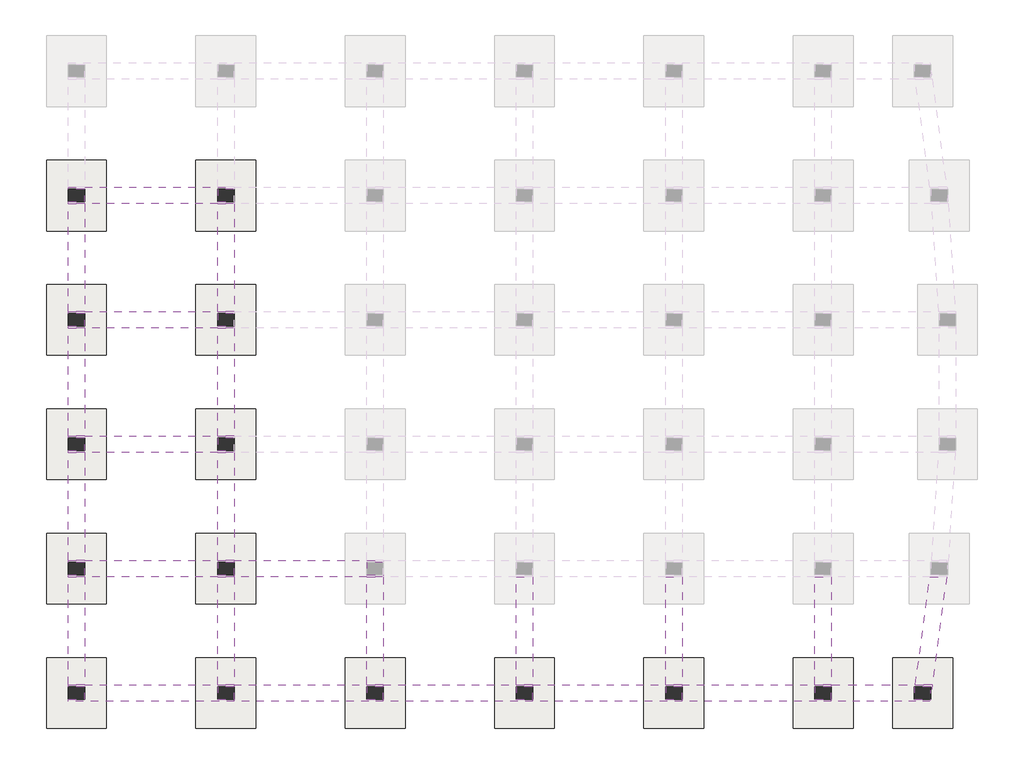
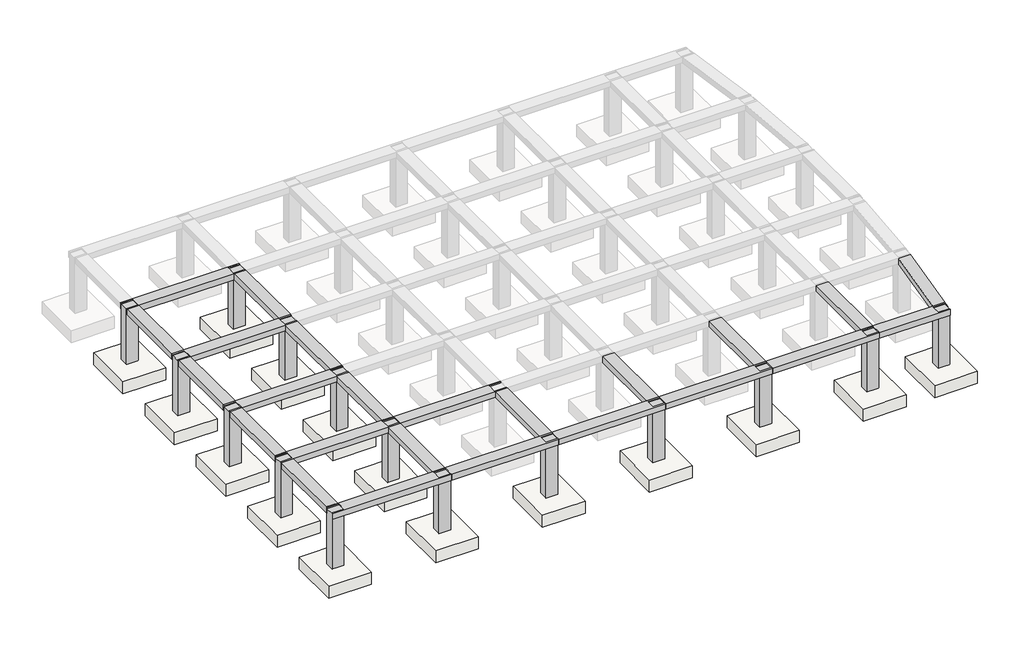
# One storey, part 1 of 3: 24 beams, 15 columns, 15 slabs.
"""IFC4 building model written with IfcOpenShell, lengths in millimetres."""

from ifc_helpers import new_model, si_unit, frame, origin, place, context, project, spatial, polyline, outline, extrude, faceted_brep, element, save

model = new_model("IFC4")

# Units and contexts
model_context = context("Model", 3, world=origin())
ifc_project = project(units=[si_unit("LENGTHUNIT", "METRE", prefix="MILLI")], contexts=[model_context])

# Site, building, storey
site = spatial("IfcSite", under=ifc_project)
building = spatial("IfcBuilding", under=site)
storey = spatial("IfcBuildingStorey", under=building, Elevation=-2999.978125)

# Beams
placement = place(None, origin())
element("IfcBeam", 1, ObjectType="Concrete-Rectangular Beam : 2' x2'", at=placement, inside=storey, context=model_context, shape_type="Brep", body=[
    faceted_brep([(-16619.274232, -2891.2168778, 48.021875), (-17228.874232, -2891.2168778, 48.021875), (-22105.674232, -2891.2168778, 48.021875), (-22715.274232, -2891.2168778, 48.021875), (-22715.274232, -2967.4168778, 48.021875), (-22105.674232, -2967.4168778, 48.021875), (-22105.674232, -3424.6168778, 48.021875), (-22715.274232, -3424.6168778, 48.021875), (-22715.274232, -3500.8168778, 48.021875), (-16619.274232, -3500.8168778, 48.021875), (-16619.274232, -3424.6168778, 48.021875), (-17228.874232, -3424.6168778, 48.021875), (-17228.874232, -2967.4168778, 48.021875), (-16619.274232, -2967.4168778, 48.021875), (-22715.274232, -3500.8168778, -256.778125), (-16619.274232, -3500.8168778, -256.778125), (-17228.874232, -3424.6168778, -256.778125), (-16619.274232, -3424.6168778, -256.778125), (-22715.274232, -3424.6168778, -256.778125), (-22105.674232, -3424.6168778, -256.778125), (-22105.674232, -2967.4168778, -256.778125), (-22715.274232, -2967.4168778, -256.778125), (-22715.274232, -2891.2168778, -256.778125), (-22105.674232, -2891.2168778, -256.778125), (-17228.874232, -2891.2168778, -256.778125), (-16619.274232, -2891.2168778, -256.778125), (-16619.274232, -2967.4168778, -256.778125), (-17228.874232, -2967.4168778, -256.778125)], [[[0, 1, 2, 3, 4, 5, 6, 7, 8, 9, 10, 11, 12, 13]], [[8, 14, 15, 9]], [[16, 17, 15, 14, 18, 19, 20, 21, 22, 23, 24, 25, 26, 27]], [[22, 3, 2, 1, 0, 25, 24, 23]], [[20, 19, 6, 5]], [[19, 18, 7, 6]], [[21, 20, 5, 4]], [[11, 10, 17, 16]], [[11, 16, 27, 12]], [[12, 27, 26, 13]], [[14, 8, 7, 18]], [[9, 15, 17, 10]], [[3, 22, 21, 4]], [[25, 0, 13, 26]]]),
])
element("IfcBeam", 2, ObjectType="Concrete-Rectangular Beam : 2' x2'", at=placement, inside=storey, context=model_context, shape_type="Brep", body=[
    faceted_brep([(-16619.274232, -2891.2168778, 48.021875), (-16619.274232, -2967.4168778, 48.021875), (-16619.274232, -3424.6168778, 48.021875), (-16619.274232, -3500.8168778, 48.021875), (-11132.874232, -3500.8168778, 48.021875), (-11132.874232, -3424.6168778, 48.021875), (-11742.474232, -3424.6168778, 48.021875), (-11742.474232, -2967.4168778, 48.021875), (-11132.874232, -2967.4168778, 48.021875), (-11132.874232, -2891.2168778, 48.021875), (-11742.474232, -2891.2168778, 48.021875), (-11132.874232, -3500.8168778, -256.778125), (-16619.274232, -3500.8168778, -256.778125), (-16619.274232, -3424.6168778, -256.778125), (-16619.274232, -2967.4168778, -256.778125), (-16619.274232, -2891.2168778, -256.778125), (-11742.474232, -2891.2168778, -256.778125), (-11132.874232, -2891.2168778, -256.778125), (-11132.874232, -2967.4168778, -256.778125), (-11742.474232, -2967.4168778, -256.778125), (-11742.474232, -3424.6168778, -256.778125), (-11132.874232, -3424.6168778, -256.778125)], [[[0, 1, 2, 3, 4, 5, 6, 7, 8, 9, 10]], [[11, 4, 3, 12]], [[12, 13, 14, 15, 16, 17, 18, 19, 20, 21, 11]], [[15, 0, 10, 9, 17, 16]], [[3, 2, 1, 0, 15, 14, 13, 12]], [[6, 5, 21, 20]], [[6, 20, 19, 7]], [[7, 19, 18, 8]], [[4, 11, 21, 5]], [[17, 9, 8, 18]]]),
])
element("IfcBeam", 3, ObjectType="Concrete-Rectangular Beam : 2' x2'", at=placement, inside=storey, context=model_context, shape_type="Brep", body=[
    faceted_brep([(-5646.474232, -2891.2168778, 48.021875), (-6256.074232, -2891.2168778, 48.021875), (-11132.874232, -2891.2168778, 48.021875), (-11132.874232, -2967.4168778, 48.021875), (-11132.874232, -3424.6168778, 48.021875), (-11132.874232, -3500.8168778, 48.021875), (-5646.474232, -3500.8168778, 48.021875), (-5646.474232, -3424.6168778, 48.021875), (-6256.074232, -3424.6168778, 48.021875), (-6256.074232, -2967.4168778, 48.021875), (-5646.474232, -2967.4168778, 48.021875), (-5646.474232, -3500.8168778, -256.778125), (-11132.874232, -3500.8168778, -256.778125), (-6256.074232, -3424.6168778, -256.778125), (-5646.474232, -3424.6168778, -256.778125), (-11132.874232, -3424.6168778, -256.778125), (-11132.874232, -2967.4168778, -256.778125), (-11132.874232, -2891.2168778, -256.778125), (-6256.074232, -2891.2168778, -256.778125), (-5646.474232, -2891.2168778, -256.778125), (-5646.474232, -2967.4168778, -256.778125), (-6256.074232, -2967.4168778, -256.778125)], [[[0, 1, 2, 3, 4, 5, 6, 7, 8, 9, 10]], [[11, 6, 5, 12]], [[13, 14, 11, 12, 15, 16, 17, 18, 19, 20, 21]], [[0, 19, 18, 17, 2, 1]], [[5, 4, 3, 2, 17, 16, 15, 12]], [[8, 7, 14, 13]], [[8, 13, 21, 9]], [[9, 21, 20, 10]], [[6, 11, 14, 7]], [[19, 0, 10, 20]]]),
])
element("IfcBeam", 4, ObjectType="Concrete-Rectangular Beam : 2' x2'", at=placement, inside=storey, context=model_context, shape_type="Brep", body=[
    faceted_brep([(-5646.474232, -2891.2168778, 48.021875), (-5646.474232, -2967.4168778, 48.021875), (-5646.474232, -3424.6168778, 48.021875), (-5646.474232, -3500.8168778, 48.021875), (-160.074232, -3500.8168778, 48.021875), (-160.074232, -3424.6168778, 48.021875), (-769.674232, -3424.6168778, 48.021875), (-769.674232, -2967.4168778, 48.021875), (-160.074232, -2967.4168778, 48.021875), (-160.074232, -2891.2168778, 48.021875), (-769.674232, -2891.2168778, 48.021875), (-160.074232, -3500.8168778, -256.778125), (-5646.474232, -3500.8168778, -256.778125), (-5646.474232, -3424.6168778, -256.778125), (-5646.474232, -2967.4168778, -256.778125), (-5646.474232, -2891.2168778, -256.778125), (-769.674232, -2891.2168778, -256.778125), (-160.074232, -2891.2168778, -256.778125), (-160.074232, -2967.4168778, -256.778125), (-769.674232, -2967.4168778, -256.778125), (-769.674232, -3424.6168778, -256.778125), (-160.074232, -3424.6168778, -256.778125)], [[[0, 1, 2, 3, 4, 5, 6, 7, 8, 9, 10]], [[11, 4, 3, 12]], [[12, 13, 14, 15, 16, 17, 18, 19, 20, 21, 11]], [[15, 0, 10, 9, 17, 16]], [[3, 2, 1, 0, 15, 14, 13, 12]], [[6, 5, 21, 20]], [[6, 20, 19, 7]], [[7, 19, 18, 8]], [[4, 11, 21, 5]], [[17, 9, 8, 18]]]),
])
element("IfcBeam", 5, ObjectType="Concrete-Rectangular Beam : 2' x2'", at=placement, inside=storey, context=model_context, shape_type="Brep", body=[
    faceted_brep([(-160.074232, -2891.2168778, 48.021875), (-160.074232, -2967.4168778, 48.021875), (-160.074232, -3424.6168778, 48.021875), (-160.074232, -3500.8168778, 48.021875), (5326.325768, -3500.8168778, 48.021875), (5326.325768, -3424.6168778, 48.021875), (4716.725768, -3424.6168778, 48.021875), (4716.725768, -2967.4168778, 48.021875), (5326.325768, -2967.4168778, 48.021875), (5326.325768, -2891.2168778, 48.021875), (4716.725768, -2891.2168778, 48.021875), (5326.325768, -3500.8168778, -256.778125), (-160.074232, -3500.8168778, -256.778125), (-160.074232, -3424.6168778, -256.778125), (-160.074232, -2967.4168778, -256.778125), (-160.074232, -2891.2168778, -256.778125), (4716.725768, -2891.2168778, -256.778125), (5326.325768, -2891.2168778, -256.778125), (5326.325768, -2967.4168778, -256.778125), (4716.725768, -2967.4168778, -256.778125), (4716.725768, -3424.6168778, -256.778125), (5326.325768, -3424.6168778, -256.778125)], [[[0, 1, 2, 3, 4, 5, 6, 7, 8, 9, 10]], [[11, 4, 3, 12]], [[12, 13, 14, 15, 16, 17, 18, 19, 20, 21, 11]], [[15, 0, 10, 9, 17, 16]], [[3, 2, 1, 0, 15, 14, 13, 12]], [[6, 5, 21, 20]], [[6, 20, 19, 7]], [[7, 19, 18, 8]], [[4, 11, 21, 5]], [[17, 9, 8, 18]]]),
])
element("IfcBeam", 6, ObjectType="Concrete-Rectangular Beam : 2' x2'", at=placement, inside=storey, context=model_context, shape_type="Brep", body=[
    faceted_brep([(9027.2344863, -2891.2168778, 48.021875), (8412.2463849, -2891.2168778, 48.021875), (5326.325768, -2891.2168778, 48.021875), (5326.325768, -2967.4168778, 48.021875), (5326.325768, -3424.6168778, 48.021875), (5326.325768, -3500.8168778, 48.021875), (8946.005151, -3500.8168778, 48.021875), (8956.158818, -3424.6168778, 48.021875), (8374.325768, -3424.6168778, 48.021875), (8374.325768, -2967.4168778, 48.021875), (8983.925768, -2967.4168778, 48.021875), (8983.925768, -3216.2348608, 48.021875), (8946.005151, -3500.8168778, -256.778125), (5326.325768, -3500.8168778, -256.778125), (8374.325768, -3424.6168778, -256.778125), (8956.158818, -3424.6168778, -256.778125), (5326.325768, -3424.6168778, -256.778125), (5326.325768, -2967.4168778, -256.778125), (5326.325768, -2891.2168778, -256.778125), (8412.2463849, -2891.2168778, -256.778125), (9027.2344863, -2891.2168778, -256.778125), (8983.925768, -3216.2348608, -256.778125), (8983.925768, -2967.4168778, -256.778125), (8374.325768, -2967.4168778, -256.778125)], [[[0, 1, 2, 3, 4, 5, 6, 7, 8, 9, 10, 11]], [[12, 6, 5, 13]], [[14, 15, 12, 13, 16, 17, 18, 19, 20, 21, 22, 23]], [[0, 20, 19, 18, 2, 1]], [[5, 4, 3, 2, 18, 17, 16, 13]], [[8, 7, 15, 14]], [[8, 14, 23, 9]], [[9, 23, 22, 10]], [[6, 12, 15, 7]], [[10, 22, 21, 11]], [[20, 0, 11, 21]]]),
])
element("IfcBeam", 7, ObjectType="Concrete-Rectangular Beam : 2' x2'", at=placement, inside=storey, context=model_context, shape_type="Brep", body=[
    faceted_brep([(-16619.274232, 1680.7831222, 48.021875), (-17228.874232, 1680.7831222, 48.021875), (-22105.674232, 1680.7831222, 48.021875), (-22715.274232, 1680.7831222, 48.021875), (-22715.274232, 1604.5831222, 48.021875), (-22105.674232, 1604.5831222, 48.021875), (-22105.674232, 1147.3831222, 48.021875), (-22715.274232, 1147.3831222, 48.021875), (-22715.274232, 1071.1831222, 48.021875), (-22105.674232, 1071.1831222, 48.021875), (-17228.874232, 1071.1831222, 48.021875), (-16619.274232, 1071.1831222, 48.021875), (-16619.274232, 1147.3831222, 48.021875), (-17228.874232, 1147.3831222, 48.021875), (-17228.874232, 1604.5831222, 48.021875), (-16619.274232, 1604.5831222, 48.021875), (-22715.274232, 1071.1831222, -256.778125), (-22105.674232, 1071.1831222, -256.778125), (-17228.874232, 1071.1831222, -256.778125), (-16619.274232, 1071.1831222, -256.778125), (-17228.874232, 1147.3831222, -256.778125), (-16619.274232, 1147.3831222, -256.778125), (-22715.274232, 1147.3831222, -256.778125), (-22105.674232, 1147.3831222, -256.778125), (-22105.674232, 1604.5831222, -256.778125), (-22715.274232, 1604.5831222, -256.778125), (-22715.274232, 1680.7831222, -256.778125), (-22105.674232, 1680.7831222, -256.778125), (-17228.874232, 1680.7831222, -256.778125), (-16619.274232, 1680.7831222, -256.778125), (-16619.274232, 1604.5831222, -256.778125), (-17228.874232, 1604.5831222, -256.778125)], [[[0, 1, 2, 3, 4, 5, 6, 7, 8, 9, 10, 11, 12, 13, 14, 15]], [[8, 16, 17, 18, 19, 11, 10, 9]], [[20, 21, 19, 18, 17, 16, 22, 23, 24, 25, 26, 27, 28, 29, 30, 31]], [[26, 3, 2, 1, 0, 29, 28, 27]], [[24, 23, 6, 5]], [[23, 22, 7, 6]], [[25, 24, 5, 4]], [[13, 12, 21, 20]], [[13, 20, 31, 14]], [[14, 31, 30, 15]], [[16, 8, 7, 22]], [[11, 19, 21, 12]], [[3, 26, 25, 4]], [[29, 0, 15, 30]]]),
])
element("IfcBeam", 8, ObjectType="Concrete-Rectangular Beam : 2' x2'", at=placement, inside=storey, context=model_context, shape_type="Brep", body=[
    faceted_brep([(-16619.274232, 1680.7831222, 48.021875), (-16619.274232, 1604.5831222, 48.021875), (-16619.274232, 1147.3831222, 48.021875), (-16619.274232, 1071.1831222, 48.021875), (-11742.474232, 1071.1831222, 48.021875), (-11132.874232, 1071.1831222, 48.021875), (-11132.874232, 1147.3831222, 48.021875), (-11742.474232, 1147.3831222, 48.021875), (-11742.474232, 1604.5831222, 48.021875), (-11132.874232, 1604.5831222, 48.021875), (-11132.874232, 1680.7831222, 48.021875), (-11742.474232, 1680.7831222, 48.021875), (-16619.274232, 1071.1831222, -256.778125), (-11742.474232, 1071.1831222, -256.778125), (-11132.874232, 1071.1831222, -256.778125), (-11742.474232, 1147.3831222, -256.778125), (-11132.874232, 1147.3831222, -256.778125), (-16619.274232, 1147.3831222, -256.778125), (-16619.274232, 1604.5831222, -256.778125), (-16619.274232, 1680.7831222, -256.778125), (-11742.474232, 1680.7831222, -256.778125), (-11132.874232, 1680.7831222, -256.778125), (-11132.874232, 1604.5831222, -256.778125), (-11742.474232, 1604.5831222, -256.778125)], [[[0, 1, 2, 3, 4, 5, 6, 7, 8, 9, 10, 11]], [[3, 12, 13, 14, 5, 4]], [[15, 16, 14, 13, 12, 17, 18, 19, 20, 21, 22, 23]], [[10, 21, 20, 19, 0, 11]], [[3, 2, 1, 0, 19, 18, 17, 12]], [[7, 6, 16, 15]], [[7, 15, 23, 8]], [[8, 23, 22, 9]], [[5, 14, 16, 6]], [[21, 10, 9, 22]]]),
])
element("IfcBeam", 9, ObjectType="Concrete-Rectangular Beam : 2' x2'", at=placement, inside=storey, context=model_context, shape_type="Brep", body=[
    faceted_brep([(-16619.274232, 6252.7831222, 48.021875), (-17228.874232, 6252.7831222, 48.021875), (-22105.674232, 6252.7831222, 48.021875), (-22715.274232, 6252.7831222, 48.021875), (-22715.274232, 6176.5831222, 48.021875), (-22105.674232, 6176.5831222, 48.021875), (-22105.674232, 5719.3831222, 48.021875), (-22715.274232, 5719.3831222, 48.021875), (-22715.274232, 5643.1831222, 48.021875), (-22105.674232, 5643.1831222, 48.021875), (-17228.874232, 5643.1831222, 48.021875), (-16619.274232, 5643.1831222, 48.021875), (-16619.274232, 5719.3831222, 48.021875), (-17228.874232, 5719.3831222, 48.021875), (-17228.874232, 6176.5831222, 48.021875), (-16619.274232, 6176.5831222, 48.021875), (-22715.274232, 5643.1831222, -256.778125), (-22105.674232, 5643.1831222, -256.778125), (-17228.874232, 5643.1831222, -256.778125), (-16619.274232, 5643.1831222, -256.778125), (-17228.874232, 5719.3831222, -256.778125), (-16619.274232, 5719.3831222, -256.778125), (-22715.274232, 5719.3831222, -256.778125), (-22105.674232, 5719.3831222, -256.778125), (-22105.674232, 6176.5831222, -256.778125), (-22715.274232, 6176.5831222, -256.778125), (-22715.274232, 6252.7831222, -256.778125), (-22105.674232, 6252.7831222, -256.778125), (-17228.874232, 6252.7831222, -256.778125), (-16619.274232, 6252.7831222, -256.778125), (-16619.274232, 6176.5831222, -256.778125), (-17228.874232, 6176.5831222, -256.778125)], [[[0, 1, 2, 3, 4, 5, 6, 7, 8, 9, 10, 11, 12, 13, 14, 15]], [[8, 16, 17, 18, 19, 11, 10, 9]], [[20, 21, 19, 18, 17, 16, 22, 23, 24, 25, 26, 27, 28, 29, 30, 31]], [[26, 3, 2, 1, 0, 29, 28, 27]], [[24, 23, 6, 5]], [[23, 22, 7, 6]], [[25, 24, 5, 4]], [[13, 12, 21, 20]], [[13, 20, 31, 14]], [[14, 31, 30, 15]], [[16, 8, 7, 22]], [[11, 19, 21, 12]], [[3, 26, 25, 4]], [[29, 0, 15, 30]]]),
])
element("IfcBeam", 10, ObjectType="Concrete-Rectangular Beam : 2' x2'", at=placement, inside=storey, context=model_context, shape_type="Brep", body=[
    faceted_brep([(-16619.274232, 10824.7831222, 48.021875), (-17228.874232, 10824.7831222, 48.021875), (-22105.674232, 10824.7831222, 48.021875), (-22715.274232, 10824.7831222, 48.021875), (-22715.274232, 10748.5831222, 48.021875), (-22105.674232, 10748.5831222, 48.021875), (-22105.674232, 10291.3831222, 48.021875), (-22715.274232, 10291.3831222, 48.021875), (-22715.274232, 10215.1831222, 48.021875), (-22105.674232, 10215.1831222, 48.021875), (-17228.874232, 10215.1831222, 48.021875), (-16619.274232, 10215.1831222, 48.021875), (-16619.274232, 10291.3831222, 48.021875), (-17228.874232, 10291.3831222, 48.021875), (-17228.874232, 10748.5831222, 48.021875), (-16619.274232, 10748.5831222, 48.021875), (-22715.274232, 10215.1831222, -256.778125), (-22105.674232, 10215.1831222, -256.778125), (-17228.874232, 10215.1831222, -256.778125), (-16619.274232, 10215.1831222, -256.778125), (-17228.874232, 10291.3831222, -256.778125), (-16619.274232, 10291.3831222, -256.778125), (-22715.274232, 10291.3831222, -256.778125), (-22105.674232, 10291.3831222, -256.778125), (-22105.674232, 10748.5831222, -256.778125), (-22715.274232, 10748.5831222, -256.778125), (-22715.274232, 10824.7831222, -256.778125), (-22105.674232, 10824.7831222, -256.778125), (-17228.874232, 10824.7831222, -256.778125), (-16619.274232, 10824.7831222, -256.778125), (-16619.274232, 10748.5831222, -256.778125), (-17228.874232, 10748.5831222, -256.778125)], [[[0, 1, 2, 3, 4, 5, 6, 7, 8, 9, 10, 11, 12, 13, 14, 15]], [[8, 16, 17, 18, 19, 11, 10, 9]], [[20, 21, 19, 18, 17, 16, 22, 23, 24, 25, 26, 27, 28, 29, 30, 31]], [[26, 3, 2, 1, 0, 29, 28, 27]], [[24, 23, 6, 5]], [[23, 22, 7, 6]], [[25, 24, 5, 4]], [[13, 12, 21, 20]], [[13, 20, 31, 14]], [[14, 31, 30, 15]], [[16, 8, 7, 22]], [[11, 19, 21, 12]], [[3, 26, 25, 4]], [[29, 0, 15, 30]]]),
])
element("IfcBeam", 11, ObjectType="Concrete-Rectangular Beam : 2' x2'", at=placement, inside=storey, context=model_context, shape_type="Brep", body=[
    faceted_brep([(-16619.274232, 15396.7831222, 48.021875), (-17228.874232, 15396.7831222, 48.021875), (-22105.674232, 15396.7831222, 48.021875), (-22715.274232, 15396.7831222, 48.021875), (-22715.274232, 15320.5831222, 48.021875), (-22105.674232, 15320.5831222, 48.021875), (-22105.674232, 14863.3831222, 48.021875), (-22715.274232, 14863.3831222, 48.021875), (-22715.274232, 14787.1831222, 48.021875), (-22105.674232, 14787.1831222, 48.021875), (-17228.874232, 14787.1831222, 48.021875), (-16619.274232, 14787.1831222, 48.021875), (-16619.274232, 14863.3831222, 48.021875), (-17228.874232, 14863.3831222, 48.021875), (-17228.874232, 15320.5831222, 48.021875), (-16619.274232, 15320.5831222, 48.021875), (-22715.274232, 14787.1831222, -256.778125), (-22105.674232, 14787.1831222, -256.778125), (-17228.874232, 14787.1831222, -256.778125), (-16619.274232, 14787.1831222, -256.778125), (-17228.874232, 14863.3831222, -256.778125), (-16619.274232, 14863.3831222, -256.778125), (-22715.274232, 14863.3831222, -256.778125), (-22105.674232, 14863.3831222, -256.778125), (-22105.674232, 15320.5831222, -256.778125), (-22715.274232, 15320.5831222, -256.778125), (-22715.274232, 15396.7831222, -256.778125), (-22105.674232, 15396.7831222, -256.778125), (-17228.874232, 15396.7831222, -256.778125), (-16619.274232, 15396.7831222, -256.778125), (-16619.274232, 15320.5831222, -256.778125), (-17228.874232, 15320.5831222, -256.778125)], [[[0, 1, 2, 3, 4, 5, 6, 7, 8, 9, 10, 11, 12, 13, 14, 15]], [[8, 16, 17, 18, 19, 11, 10, 9]], [[20, 21, 19, 18, 17, 16, 22, 23, 24, 25, 26, 27, 28, 29, 30, 31]], [[26, 3, 2, 1, 0, 29, 28, 27]], [[24, 23, 6, 5]], [[23, 22, 7, 6]], [[25, 24, 5, 4]], [[13, 12, 21, 20]], [[13, 20, 31, 14]], [[14, 31, 30, 15]], [[16, 8, 7, 22]], [[11, 19, 21, 12]], [[3, 26, 25, 4]], [[29, 0, 15, 30]]]),
])
element("IfcBeam", 12, ObjectType="Concrete-Rectangular Beam : 2' x2'", at=placement, inside=storey, context=model_context, shape_type="SweptSolid", body=[
    extrude(outline(polyline([(-22105.674232, -2891.2168778), (-22715.274232, -2891.2168778), (-22715.274232, 1071.1831222), (-22105.674232, 1071.1831222), (-22105.674232, -2891.2168778)])), frame((0.0, 0.0, -256.778125), z_axis=(0.0, 0.0, 1.0), x_axis=(1.0, 0.0, 0.0)), (0.0, 0.0, 1.0), 304.8),
])
element("IfcBeam", 13, ObjectType="Concrete-Rectangular Beam : 2' x2'", at=placement, inside=storey, context=model_context, shape_type="SweptSolid", body=[
    extrude(outline(polyline([(-22105.674232, 1680.7831222), (-22715.274232, 1680.7831222), (-22715.274232, 5643.1831222), (-22105.674232, 5643.1831222), (-22105.674232, 1680.7831222)])), frame((0.0, 0.0, -256.778125), z_axis=(0.0, 0.0, 1.0), x_axis=(1.0, 0.0, 0.0)), (0.0, 0.0, 1.0), 304.8),
])
element("IfcBeam", 14, ObjectType="Concrete-Rectangular Beam : 2' x2'", at=placement, inside=storey, context=model_context, shape_type="SweptSolid", body=[
    extrude(outline(polyline([(-22105.674232, 6252.7831222), (-22715.274232, 6252.7831222), (-22715.274232, 10215.1831222), (-22105.674232, 10215.1831222), (-22105.674232, 6252.7831222)])), frame((0.0, 0.0, -256.778125), z_axis=(0.0, 0.0, 1.0), x_axis=(1.0, 0.0, 0.0)), (0.0, 0.0, 1.0), 304.8),
])
element("IfcBeam", 15, ObjectType="Concrete-Rectangular Beam : 2' x2'", at=placement, inside=storey, context=model_context, shape_type="SweptSolid", body=[
    extrude(outline(polyline([(-22105.674232, 10824.7831222), (-22715.274232, 10824.7831222), (-22715.274232, 14787.1831222), (-22105.674232, 14787.1831222), (-22105.674232, 10824.7831222)])), frame((0.0, 0.0, -256.778125), z_axis=(0.0, 0.0, 1.0), x_axis=(1.0, 0.0, 0.0)), (0.0, 0.0, 1.0), 304.8),
])
element("IfcBeam", 16, ObjectType="Concrete-Rectangular Beam : 2' x2'", at=placement, inside=storey, context=model_context, shape_type="SweptSolid", body=[
    extrude(outline(polyline([(-17228.874232, 1071.1831222), (-16619.274232, 1071.1831222), (-16619.274232, -2891.2168778), (-17228.874232, -2891.2168778), (-17228.874232, 1071.1831222)])), frame((0.0, 0.0, -256.778125), z_axis=(0.0, 0.0, 1.0), x_axis=(1.0, 0.0, 0.0)), (0.0, 0.0, 1.0), 304.8),
])
element("IfcBeam", 17, ObjectType="Concrete-Rectangular Beam : 2' x2'", at=placement, inside=storey, context=model_context, shape_type="SweptSolid", body=[
    extrude(outline(polyline([(-16619.274232, 1680.7831222), (-17228.874232, 1680.7831222), (-17228.874232, 5643.1831222), (-16619.274232, 5643.1831222), (-16619.274232, 1680.7831222)])), frame((0.0, 0.0, -256.778125), z_axis=(0.0, 0.0, 1.0), x_axis=(1.0, 0.0, 0.0)), (0.0, 0.0, 1.0), 304.8),
])
element("IfcBeam", 18, ObjectType="Concrete-Rectangular Beam : 2' x2'", at=placement, inside=storey, context=model_context, shape_type="SweptSolid", body=[
    extrude(outline(polyline([(-16619.274232, 6252.7831222), (-17228.874232, 6252.7831222), (-17228.874232, 10215.1831222), (-16619.274232, 10215.1831222), (-16619.274232, 6252.7831222)])), frame((0.0, 0.0, -256.778125), z_axis=(0.0, 0.0, 1.0), x_axis=(1.0, 0.0, 0.0)), (0.0, 0.0, 1.0), 304.8),
])
element("IfcBeam", 19, ObjectType="Concrete-Rectangular Beam : 2' x2'", at=placement, inside=storey, context=model_context, shape_type="SweptSolid", body=[
    extrude(outline(polyline([(-16619.274232, 10824.7831222), (-17228.874232, 10824.7831222), (-17228.874232, 14787.1831222), (-16619.274232, 14787.1831222), (-16619.274232, 10824.7831222)])), frame((0.0, 0.0, -256.778125), z_axis=(0.0, 0.0, 1.0), x_axis=(1.0, 0.0, 0.0)), (0.0, 0.0, 1.0), 304.8),
])
element("IfcBeam", 20, ObjectType="Concrete-Rectangular Beam : 2' x2'", at=placement, inside=storey, context=model_context, shape_type="SweptSolid", body=[
    extrude(outline(polyline([(-11742.474232, 1071.1831222), (-11132.874232, 1071.1831222), (-11132.874232, -2891.2168778), (-11742.474232, -2891.2168778), (-11742.474232, 1071.1831222)])), frame((0.0, 0.0, -256.778125), z_axis=(0.0, 0.0, 1.0), x_axis=(1.0, 0.0, 0.0)), (0.0, 0.0, 1.0), 304.8),
])
element("IfcBeam", 21, ObjectType="Concrete-Rectangular Beam : 2' x2'", at=placement, inside=storey, context=model_context, shape_type="SweptSolid", body=[
    extrude(outline(polyline([(-6256.074232, 1071.1831222), (-5646.474232, 1071.1831222), (-5646.474232, -2891.2168778), (-6256.074232, -2891.2168778), (-6256.074232, 1071.1831222)])), frame((0.0, 0.0, -256.778125), z_axis=(0.0, 0.0, 1.0), x_axis=(1.0, 0.0, 0.0)), (0.0, 0.0, 1.0), 304.8),
])
element("IfcBeam", 22, ObjectType="Concrete-Rectangular Beam : 2' x2'", at=placement, inside=storey, context=model_context, shape_type="SweptSolid", body=[
    extrude(outline(polyline([(-769.674232, 1071.1831222), (-160.074232, 1071.1831222), (-160.074232, -2891.2168778), (-769.674232, -2891.2168778), (-769.674232, 1071.1831222)])), frame((0.0, 0.0, -256.778125), z_axis=(0.0, 0.0, 1.0), x_axis=(1.0, 0.0, 0.0)), (0.0, 0.0, 1.0), 304.8),
])
element("IfcBeam", 23, ObjectType="Concrete-Rectangular Beam : 2' x2'", at=placement, inside=storey, context=model_context, shape_type="SweptSolid", body=[
    extrude(outline(polyline([(4716.725768, 1071.1831222), (5326.325768, 1071.1831222), (5326.325768, -2891.2168778), (4716.725768, -2891.2168778), (4716.725768, 1071.1831222)])), frame((0.0, 0.0, -256.778125), z_axis=(0.0, 0.0, 1.0), x_axis=(1.0, 0.0, 0.0)), (0.0, 0.0, 1.0), 304.8),
])
element("IfcBeam", 24, ObjectType="Concrete-Rectangular Beam : 2' x2'", at=placement, inside=storey, context=model_context, shape_type="SweptSolid", body=[
    extrude(outline(polyline([(8940.2370643, 1071.1831222), (9555.2251658, 1071.1831222), (9027.2344863, -2891.2168778), (8412.2463849, -2891.2168778), (8940.2370643, 1071.1831222)])), frame((0.0, 0.0, -256.778125), z_axis=(0.0, 0.0, 1.0), x_axis=(1.0, 0.0, 0.0)), (0.0, 0.0, 1.0), 304.8),
])

# Columns
element("IfcColumn", 25, ObjectType="Concrete-Rectangular-Column : 12 x 18", at=placement, inside=storey, context=model_context, shape_type="SweptSolid", body=[
    extrude(outline(polyline([(-22105.674232, -2967.4168778), (-22105.674232, -3424.6168778), (-22715.274232, -3424.6168778), (-22715.274232, -2967.4168778), (-22105.674232, -2967.4168778)])), frame((0.0, 0.0, -2999.978125), z_axis=(0.0, 0.0, 1.0), x_axis=(1.0, 0.0, 0.0)), (0.0, 0.0, 1.0), 2999.978125),
])
element("IfcColumn", 26, ObjectType="Concrete-Rectangular-Column : 12 x 18", at=placement, inside=storey, context=model_context, shape_type="SweptSolid", body=[
    extrude(outline(polyline([(-16619.274232, -2967.4168778), (-16619.274232, -3424.6168778), (-17228.874232, -3424.6168778), (-17228.874232, -2967.4168778), (-16619.274232, -2967.4168778)])), frame((0.0, 0.0, -2999.978125), z_axis=(0.0, 0.0, 1.0), x_axis=(1.0, 0.0, 0.0)), (0.0, 0.0, 1.0), 2999.978125),
])
element("IfcColumn", 27, ObjectType="Concrete-Rectangular-Column : 12 x 18", at=placement, inside=storey, context=model_context, shape_type="SweptSolid", body=[
    extrude(outline(polyline([(-11132.874232, -2967.4168778), (-11132.874232, -3424.6168778), (-11742.474232, -3424.6168778), (-11742.474232, -2967.4168778), (-11132.874232, -2967.4168778)])), frame((0.0, 0.0, -2999.978125), z_axis=(0.0, 0.0, 1.0), x_axis=(1.0, 0.0, 0.0)), (0.0, 0.0, 1.0), 2999.978125),
])
element("IfcColumn", 28, ObjectType="Concrete-Rectangular-Column : 12 x 18", at=placement, inside=storey, context=model_context, shape_type="SweptSolid", body=[
    extrude(outline(polyline([(-5646.474232, -2967.4168778), (-5646.474232, -3424.6168778), (-6256.074232, -3424.6168778), (-6256.074232, -2967.4168778), (-5646.474232, -2967.4168778)])), frame((0.0, 0.0, -2999.978125), z_axis=(0.0, 0.0, 1.0), x_axis=(1.0, 0.0, 0.0)), (0.0, 0.0, 1.0), 2999.978125),
])
element("IfcColumn", 29, ObjectType="Concrete-Rectangular-Column : 12 x 18", at=placement, inside=storey, context=model_context, shape_type="SweptSolid", body=[
    extrude(outline(polyline([(-160.074232, -2967.4168778), (-160.074232, -3424.6168778), (-769.674232, -3424.6168778), (-769.674232, -2967.4168778), (-160.074232, -2967.4168778)])), frame((0.0, 0.0, -2999.978125), z_axis=(0.0, 0.0, 1.0), x_axis=(1.0, 0.0, 0.0)), (0.0, 0.0, 1.0), 2999.978125),
])
element("IfcColumn", 30, ObjectType="Concrete-Rectangular-Column : 12 x 18", at=placement, inside=storey, context=model_context, shape_type="SweptSolid", body=[
    extrude(outline(polyline([(5326.325768, -2967.4168778), (5326.325768, -3424.6168778), (4716.725768, -3424.6168778), (4716.725768, -2967.4168778), (5326.325768, -2967.4168778)])), frame((0.0, 0.0, -2999.978125), z_axis=(0.0, 0.0, 1.0), x_axis=(1.0, 0.0, 0.0)), (0.0, 0.0, 1.0), 2999.978125),
])
element("IfcColumn", 31, ObjectType="Concrete-Rectangular-Column : 12 x 18", at=placement, inside=storey, context=model_context, shape_type="SweptSolid", body=[
    extrude(outline(polyline([(8983.925768, -2967.4168778), (8983.925768, -3424.6168778), (8374.325768, -3424.6168778), (8374.325768, -2967.4168778), (8983.925768, -2967.4168778)])), frame((0.0, 0.0, -2999.978125), z_axis=(0.0, 0.0, 1.0), x_axis=(1.0, 0.0, 0.0)), (0.0, 0.0, 1.0), 2999.978125),
])
element("IfcColumn", 32, ObjectType="Concrete-Rectangular-Column : 12 x 18", at=placement, inside=storey, context=model_context, shape_type="SweptSolid", body=[
    extrude(outline(polyline([(-22105.674232, 1604.5831222), (-22105.674232, 1147.3831222), (-22715.274232, 1147.3831222), (-22715.274232, 1604.5831222), (-22105.674232, 1604.5831222)])), frame((0.0, 0.0, -2999.978125), z_axis=(0.0, 0.0, 1.0), x_axis=(1.0, 0.0, 0.0)), (0.0, 0.0, 1.0), 2999.978125),
])
element("IfcColumn", 33, ObjectType="Concrete-Rectangular-Column : 12 x 18", at=placement, inside=storey, context=model_context, shape_type="SweptSolid", body=[
    extrude(outline(polyline([(-16619.274232, 1604.5831222), (-16619.274232, 1147.3831222), (-17228.874232, 1147.3831222), (-17228.874232, 1604.5831222), (-16619.274232, 1604.5831222)])), frame((0.0, 0.0, -2999.978125), z_axis=(0.0, 0.0, 1.0), x_axis=(1.0, 0.0, 0.0)), (0.0, 0.0, 1.0), 2999.978125),
])
element("IfcColumn", 34, ObjectType="Concrete-Rectangular-Column : 12 x 18", at=placement, inside=storey, context=model_context, shape_type="SweptSolid", body=[
    extrude(outline(polyline([(-22105.674232, 6176.5831222), (-22105.674232, 5719.3831222), (-22715.274232, 5719.3831222), (-22715.274232, 6176.5831222), (-22105.674232, 6176.5831222)])), frame((0.0, 0.0, -2999.978125), z_axis=(0.0, 0.0, 1.0), x_axis=(1.0, 0.0, 0.0)), (0.0, 0.0, 1.0), 2999.978125),
])
element("IfcColumn", 35, ObjectType="Concrete-Rectangular-Column : 12 x 18", at=placement, inside=storey, context=model_context, shape_type="SweptSolid", body=[
    extrude(outline(polyline([(-16619.274232, 6176.5831222), (-16619.274232, 5719.3831222), (-17228.874232, 5719.3831222), (-17228.874232, 6176.5831222), (-16619.274232, 6176.5831222)])), frame((0.0, 0.0, -2999.978125), z_axis=(0.0, 0.0, 1.0), x_axis=(1.0, 0.0, 0.0)), (0.0, 0.0, 1.0), 2999.978125),
])
element("IfcColumn", 36, ObjectType="Concrete-Rectangular-Column : 12 x 18", at=placement, inside=storey, context=model_context, shape_type="SweptSolid", body=[
    extrude(outline(polyline([(-22105.674232, 10748.5831222), (-22105.674232, 10291.3831222), (-22715.274232, 10291.3831222), (-22715.274232, 10748.5831222), (-22105.674232, 10748.5831222)])), frame((0.0, 0.0, -2999.978125), z_axis=(0.0, 0.0, 1.0), x_axis=(1.0, 0.0, 0.0)), (0.0, 0.0, 1.0), 2999.978125),
])
element("IfcColumn", 37, ObjectType="Concrete-Rectangular-Column : 12 x 18", at=placement, inside=storey, context=model_context, shape_type="SweptSolid", body=[
    extrude(outline(polyline([(-16619.274232, 10748.5831222), (-16619.274232, 10291.3831222), (-17228.874232, 10291.3831222), (-17228.874232, 10748.5831222), (-16619.274232, 10748.5831222)])), frame((0.0, 0.0, -2999.978125), z_axis=(0.0, 0.0, 1.0), x_axis=(1.0, 0.0, 0.0)), (0.0, 0.0, 1.0), 2999.978125),
])
element("IfcColumn", 38, ObjectType="Concrete-Rectangular-Column : 12 x 18", at=placement, inside=storey, context=model_context, shape_type="SweptSolid", body=[
    extrude(outline(polyline([(-22105.674232, 15320.5831222), (-22105.674232, 14863.3831222), (-22715.274232, 14863.3831222), (-22715.274232, 15320.5831222), (-22105.674232, 15320.5831222)])), frame((0.0, 0.0, -2999.978125), z_axis=(0.0, 0.0, 1.0), x_axis=(1.0, 0.0, 0.0)), (0.0, 0.0, 1.0), 2999.978125),
])
element("IfcColumn", 39, ObjectType="Concrete-Rectangular-Column : 12 x 18", at=placement, inside=storey, context=model_context, shape_type="SweptSolid", body=[
    extrude(outline(polyline([(-16619.274232, 15320.5831222), (-16619.274232, 14863.3831222), (-17228.874232, 14863.3831222), (-17228.874232, 15320.5831222), (-16619.274232, 15320.5831222)])), frame((0.0, 0.0, -2999.978125), z_axis=(0.0, 0.0, 1.0), x_axis=(1.0, 0.0, 0.0)), (0.0, 0.0, 1.0), 2999.978125),
])

# Slabs
element("IfcSlab", 40, ObjectType="Footing-Rectangular : 650 X 2200X2600", at=placement, inside=storey, context=model_context, shape_type="SweptSolid", body=[
    extrude(outline(polyline([(-21310.4855602, -1896.0032059), (-21310.4855602, -4496.0305497), (-23510.4629039, -4496.0305497), (-23510.4629039, -1896.0032059), (-21310.4855602, -1896.0032059)])), frame((0.0, 0.0, -3649.9601562), z_axis=(0.0, 0.0, 1.0), x_axis=(1.0, 0.0, 0.0)), (0.0, 0.0, 1.0), 649.9820313),
])
element("IfcSlab", 41, ObjectType="Footing-Rectangular : 650 X 2200X2600", at=placement, inside=storey, context=model_context, shape_type="SweptSolid", body=[
    extrude(outline(polyline([(-15824.0855602, -1896.0032059), (-15824.0855602, -4496.0305497), (-18024.0629039, -4496.0305497), (-18024.0629039, -1896.0032059), (-15824.0855602, -1896.0032059)])), frame((0.0, 0.0, -3649.9601562), z_axis=(0.0, 0.0, 1.0), x_axis=(1.0, 0.0, 0.0)), (0.0, 0.0, 1.0), 649.9820313),
])
element("IfcSlab", 42, ObjectType="Footing-Rectangular : 650 X 2200X2600", at=placement, inside=storey, context=model_context, shape_type="SweptSolid", body=[
    extrude(outline(polyline([(-10337.6855602, -1896.0032059), (-10337.6855602, -4496.0305497), (-12537.6629039, -4496.0305497), (-12537.6629039, -1896.0032059), (-10337.6855602, -1896.0032059)])), frame((0.0, 0.0, -3649.9601562), z_axis=(0.0, 0.0, 1.0), x_axis=(1.0, 0.0, 0.0)), (0.0, 0.0, 1.0), 649.9820313),
])
element("IfcSlab", 43, ObjectType="Footing-Rectangular : 650 X 2200X2600", at=placement, inside=storey, context=model_context, shape_type="SweptSolid", body=[
    extrude(outline(polyline([(-4851.2855602, -1896.0032059), (-4851.2855602, -4496.0305497), (-7051.2629039, -4496.0305497), (-7051.2629039, -1896.0032059), (-4851.2855602, -1896.0032059)])), frame((0.0, 0.0, -3649.9601562), z_axis=(0.0, 0.0, 1.0), x_axis=(1.0, 0.0, 0.0)), (0.0, 0.0, 1.0), 649.9820313),
])
element("IfcSlab", 44, ObjectType="Footing-Rectangular : 650 X 2200X2600", at=placement, inside=storey, context=model_context, shape_type="SweptSolid", body=[
    extrude(outline(polyline([(635.1144398, -1896.0032059), (635.1144398, -4496.0305497), (-1564.8629039, -4496.0305497), (-1564.8629039, -1896.0032059), (635.1144398, -1896.0032059)])), frame((0.0, 0.0, -3649.9601562), z_axis=(0.0, 0.0, 1.0), x_axis=(1.0, 0.0, 0.0)), (0.0, 0.0, 1.0), 649.9820313),
])
element("IfcSlab", 45, ObjectType="Footing-Rectangular : 650 X 2200X2600", at=placement, inside=storey, context=model_context, shape_type="SweptSolid", body=[
    extrude(outline(polyline([(6121.5144398, -1896.0032059), (6121.5144398, -4496.0305497), (3921.5370961, -4496.0305497), (3921.5370961, -1896.0032059), (6121.5144398, -1896.0032059)])), frame((0.0, 0.0, -3649.9601562), z_axis=(0.0, 0.0, 1.0), x_axis=(1.0, 0.0, 0.0)), (0.0, 0.0, 1.0), 649.9820313),
])
element("IfcSlab", 46, ObjectType="Footing-Rectangular : 650 X 2200X2600", at=placement, inside=storey, context=model_context, shape_type="SweptSolid", body=[
    extrude(outline(polyline([(9779.1144398, -1896.0032059), (9779.1144398, -4496.0305497), (7579.1370961, -4496.0305497), (7579.1370961, -1896.0032059), (9779.1144398, -1896.0032059)])), frame((0.0, 0.0, -3649.9601562), z_axis=(0.0, 0.0, 1.0), x_axis=(1.0, 0.0, 0.0)), (0.0, 0.0, 1.0), 649.9820313),
])
element("IfcSlab", 47, ObjectType="Footing-Rectangular : 650 X 2200X2600", at=placement, inside=storey, context=model_context, shape_type="SweptSolid", body=[
    extrude(outline(polyline([(-21310.4855602, 2675.9967941), (-21310.4855602, 75.9694503), (-23510.4629039, 75.9694503), (-23510.4629039, 2675.9967941), (-21310.4855602, 2675.9967941)])), frame((0.0, 0.0, -3649.9601562), z_axis=(0.0, 0.0, 1.0), x_axis=(1.0, 0.0, 0.0)), (0.0, 0.0, 1.0), 649.9820313),
])
element("IfcSlab", 48, ObjectType="Footing-Rectangular : 650 X 2200X2600", at=placement, inside=storey, context=model_context, shape_type="SweptSolid", body=[
    extrude(outline(polyline([(-15824.0855602, 2675.9967941), (-15824.0855602, 75.9694503), (-18024.0629039, 75.9694503), (-18024.0629039, 2675.9967941), (-15824.0855602, 2675.9967941)])), frame((0.0, 0.0, -3649.9601562), z_axis=(0.0, 0.0, 1.0), x_axis=(1.0, 0.0, 0.0)), (0.0, 0.0, 1.0), 649.9820313),
])
element("IfcSlab", 49, ObjectType="Footing-Rectangular : 650 X 2200X2600", at=placement, inside=storey, context=model_context, shape_type="SweptSolid", body=[
    extrude(outline(polyline([(-21310.4855602, 7247.9967941), (-21310.4855602, 4647.9694503), (-23510.4629039, 4647.9694503), (-23510.4629039, 7247.9967941), (-21310.4855602, 7247.9967941)])), frame((0.0, 0.0, -3649.9601562), z_axis=(0.0, 0.0, 1.0), x_axis=(1.0, 0.0, 0.0)), (0.0, 0.0, 1.0), 649.9820313),
])
element("IfcSlab", 50, ObjectType="Footing-Rectangular : 650 X 2200X2600", at=placement, inside=storey, context=model_context, shape_type="SweptSolid", body=[
    extrude(outline(polyline([(-15824.0855602, 7247.9967941), (-15824.0855602, 4647.9694503), (-18024.0629039, 4647.9694503), (-18024.0629039, 7247.9967941), (-15824.0855602, 7247.9967941)])), frame((0.0, 0.0, -3649.9601562), z_axis=(0.0, 0.0, 1.0), x_axis=(1.0, 0.0, 0.0)), (0.0, 0.0, 1.0), 649.9820313),
])
element("IfcSlab", 51, ObjectType="Footing-Rectangular : 650 X 2200X2600", at=placement, inside=storey, context=model_context, shape_type="SweptSolid", body=[
    extrude(outline(polyline([(-21310.4855602, 11819.9967941), (-21310.4855602, 9219.9694503), (-23510.4629039, 9219.9694503), (-23510.4629039, 11819.9967941), (-21310.4855602, 11819.9967941)])), frame((0.0, 0.0, -3649.9601562), z_axis=(0.0, 0.0, 1.0), x_axis=(1.0, 0.0, 0.0)), (0.0, 0.0, 1.0), 649.9820313),
])
element("IfcSlab", 52, ObjectType="Footing-Rectangular : 650 X 2200X2600", at=placement, inside=storey, context=model_context, shape_type="SweptSolid", body=[
    extrude(outline(polyline([(-15824.0855602, 11819.9967941), (-15824.0855602, 9219.9694503), (-18024.0629039, 9219.9694503), (-18024.0629039, 11819.9967941), (-15824.0855602, 11819.9967941)])), frame((0.0, 0.0, -3649.9601562), z_axis=(0.0, 0.0, 1.0), x_axis=(1.0, 0.0, 0.0)), (0.0, 0.0, 1.0), 649.9820313),
])
element("IfcSlab", 53, ObjectType="Footing-Rectangular : 650 X 2200X2600", at=placement, inside=storey, context=model_context, shape_type="SweptSolid", body=[
    extrude(outline(polyline([(-21310.4855602, 16391.9967941), (-21310.4855602, 13791.9694503), (-23510.4629039, 13791.9694503), (-23510.4629039, 16391.9967941), (-21310.4855602, 16391.9967941)])), frame((0.0, 0.0, -3649.9601562), z_axis=(0.0, 0.0, 1.0), x_axis=(1.0, 0.0, 0.0)), (0.0, 0.0, 1.0), 649.9820313),
])
element("IfcSlab", 54, ObjectType="Footing-Rectangular : 650 X 2200X2600", at=placement, inside=storey, context=model_context, shape_type="SweptSolid", body=[
    extrude(outline(polyline([(-15824.0855602, 16391.9967941), (-15824.0855602, 13791.9694503), (-18024.0629039, 13791.9694503), (-18024.0629039, 16391.9967941), (-15824.0855602, 16391.9967941)])), frame((0.0, 0.0, -3649.9601562), z_axis=(0.0, 0.0, 1.0), x_axis=(1.0, 0.0, 0.0)), (0.0, 0.0, 1.0), 649.9820313),
])

save(model, "model.ifc")

# Revit data of these elements
# Grids (mm)
#   "3": line (11252.408, 5947.983) -> (-25304.32, 5947.983)
#   "4": line (11252.408, 10519.983) -> (-25304.32, 10519.983)
#   "1": line (11252.408, -3196.017) -> (-25304.32, -3196.017)
#   "2": line (11252.408, 1375.983) -> (-25304.32, 1375.983)
#   "5": line (11252.408, 15091.983) -> (-25304.32, 15091.983)
#   "6": line (11252.408, 19663.983) -> (-25304.32, 19663.983)
#   "A": line (-22410.474, 23675.517) -> (-22410.474, -5037.756)
#   "B": line (-16924.074, 23675.517) -> (-16924.074, -5037.756)
#   "C": line (-22410.474, 23675.517) -> (-22410.474, -5037.756)
#   "D": line (-11437.674, 23675.517) -> (-11437.674, -5037.756)
#   "E": line (-5951.274, 23675.517) -> (-5951.274, -5037.756)
#   "F": line (-464.874, 23675.517) -> (-464.874, -5037.756)
#   "G": line (5021.526, 23675.517) -> (5021.526, -5037.756)
#   "H": arc centre (-59639.039, 8233.983) radius 69267.717 angles 6.090393 to 6.495912 rad from (1, 0)
# Type "Concrete-Rectangular Beam : 2' x2'"
#   Assembly Code = "B10"
#   Length [instance default] = 5' - 0"
#   b = 2' - 0"
#   h = 1' - 0"
#   Structural Material [instance default] = Concrete, Cast-in-Place gray
# Type "Concrete-Rectangular-Column : 12 x 18"
#   Assembly Code = "B10"
#   b = 2' - 0"
#   h = 1' - 6"
#   Structural Material [instance default] = Concrete, Cast-in-Place gray
# Type "Footing-Rectangular : 650 X 2200X2600"
#   Assembly Code = "A1010100"
#   Width = 7' - 2 157/256"
#   Length = 8' - 6 93/256"
#   Foundation Thickness = 2' - 1 151/256"
#   Structural Material [instance default] = Concrete, Cast-in-Place gray
# Elements 1, 2, 3, 4, 5, 6, 7, 8, 9, 10, 11, 12, 13, 14, 15, 16, 17, 18, 19, 20, 21, 22, 23, 24 (IfcBeam, "Concrete-Rectangular Beam : 2' x2'")
#   Structural Material = Concrete, Precast (2)
#   Phase Created = New Construction
#   Materials on its faces: "Concrete, Precast (2)"
# Elements 25, 26, 27, 28, 29, 30, 31, 32, 33, 34, 35, 36, 37, 38, 39 (IfcColumn, "Concrete-Rectangular-Column : 12 x 18")
#   Phase Created = New Construction
#   Materials on its faces: "Concrete, Cast-in-Place gray"
# Elements 40, 41, 42, 43, 44, 45, 46, 47, 48, 49, 50, 51, 52, 53, 54 (IfcSlab, "Footing-Rectangular : 650 X 2200X2600")
#   Structural Material = Concrete, Cast-in-Place gray
#   Phase Created = New Construction
#   Materials on its faces: "Concrete, Cast-in-Place gray"
# Materials
#   "Concrete, Cast-in-Place gray": class "Concrete", colour RGB 192 192 192, transparency 0, Description = "Cast-in-place concrete", Cost = 0
#   "Concrete, Precast (2)": class "Concrete", colour RGB 198 187 187, transparency 0, Description = "Precast concrete", Cost = 0
